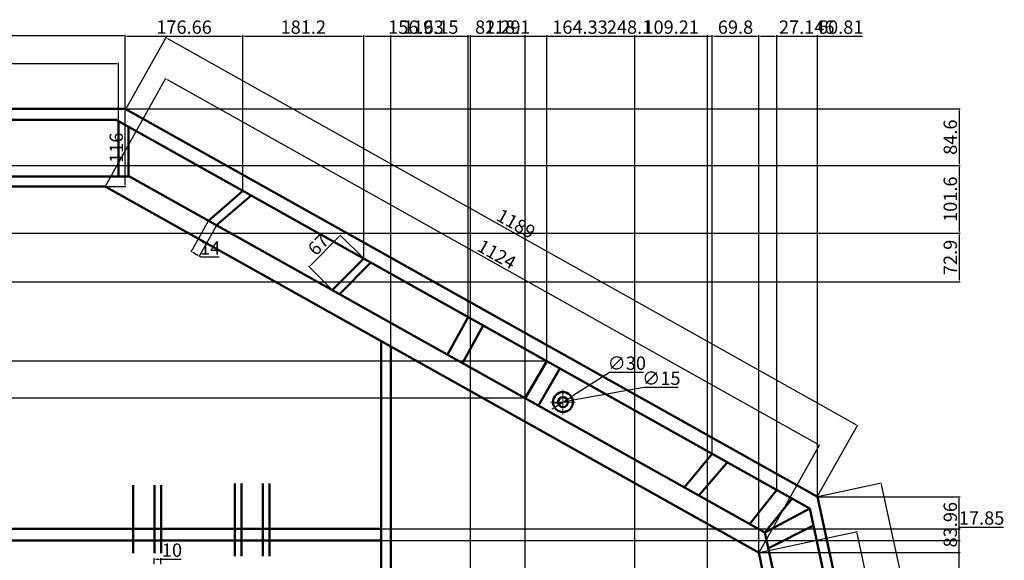
# Model space of a CAD drawing. Units: millimetres. Extents: x 1408 to 3734, y 1022 to 2569.
# Tile 3 of 3: x 2256 to 3734, y 1758 to 2569. Entities that reach past the tile are written whole.
import ezdxf

# ---------------------------------------------------------------- set-up
doc = ezdxf.new("R2010")
doc.units = ezdxf.units.MM
doc.linetypes.add('CENTER2', pattern=[28.575, 19.05, -3.175, 3.175, -3.175])
for name, color, linetype, lineweight in [('M-CNTR', 1, 'CENTER2', 18), ('M-DIMS', 2, 'Continuous', 25), ('M-OUTL', 7, 'Continuous', 50)]:
    doc.layers.add(name, color=color, linetype=linetype, lineweight=lineweight)
doc.styles.get("Standard").update_dxf_attribs({"font": 'arial.ttf'})
doc.dimstyles.new('ISO-25', dxfattribs={"dimtxt": 20, "dimasz": 2.5, "dimexe": 1.25, "dimexo": 0.625, "dimtad": 1, "dimtoh": 1, "dimdec": 0, "dimtxsty": 'Standard', "dimcen": 2.5, "dimadec": 0, "dimazin": 0, "dimtfac": 1, "dimtdec": 0, "dimtmove": 0, "dimatfit": 3, "dimfxl": 1, "dimarcsym": 0})

# ---------------------------------------------------------------- blocks, each defined once
blk = doc.blocks.new('*U1')
at = {"layer": 'M-CNTR', "color": 0, "transparency": 16777216}
for p, q in [((-11, 0), (-1.5, 0)), ((0, 1.5), (0, 11)), ((1.5, 0), (11, 0)), ((0, -11), (0, -1.5))]:
    blk.add_line(p, q, dxfattribs=at)
at = {"layer": 'M-CNTR', "color": 0, "linetype": 'Continuous', "transparency": 16777216}
for p, q in [((-0.7, 0), (0.7, 0)), ((0, -0.7), (0, 0.7))]:
    blk.add_line(p, q, dxfattribs=at)
blk = doc.blocks.new('*U2')
at = {"layer": 'M-CNTR', "color": 0, "transparency": 16777216}
for p, q in [((0, 3), (0, 18.5)), ((-18.5, 0), (-3, 0)), ((3, 0), (18.5, 0)), ((0, -18.5), (0, -3))]:
    blk.add_line(p, q, dxfattribs=at)
at = {"layer": 'M-CNTR', "color": 0, "linetype": 'Continuous', "transparency": 16777216}
for p, q in [((-1.5, 0), (1.5, 0)), ((0, -1.5), (0, 1.5))]:
    blk.add_line(p, q, dxfattribs=at)
blk = doc.blocks.new('*D10')
at = {"layer": 'Defpoints', "color": 0, "transparency": 16777216}
for p in [(2414.7, 2435.4), (2414.7, 2435.4), (2384.8, 2318.9)]:
    blk.add_point(p, dxfattribs=at)
at = {"layer": 'M-DIMS', "color": 0, "lineweight": -2, "transparency": 16777216}
for p, q in [((2414.7, 2321.4), (2414.7, 2432.9)), ((2415.3, 2435.4), (2415.9, 2435.4)), ((2385.4, 2318.9), (2415.9, 2318.9))]:
    blk.add_line(p, q, dxfattribs=at)
at = {"layer": 'M-DIMS', "color": 0, "transparency": 16777216}
for points in [[(2414.3, 2432.9), (2415.1, 2432.9), (2414.7, 2435.4)], [(2414.3, 2321.4), (2415.1, 2321.4), (2414.7, 2318.9)]]:
    blk.add_solid(points, dxfattribs=at)
at = {"layer": 'M-DIMS', "color": 0, "transparency": 16777216, "insert": (2403.9, 2377.2), "char_height": 20, "attachment_point": 5, "rotation": 90}
blk.add_mtext('116', dxfattribs=at)
blk = doc.blocks.new('*D11')
at = {"layer": 'Defpoints', "color": 0, "transparency": 16777216}
for p in [(2415.9, 2435.4), (3513.1, 1960.8), (3453.1, 1853.8)]:
    blk.add_point(p, dxfattribs=at)
at = {"layer": 'M-DIMS', "color": 0, "lineweight": -2, "transparency": 16777216}
for p, q in [((2416.3, 2435.9), (2476.5, 2543.4)), ((2478.1, 2541.1), (3510.9, 1962)), ((3453.4, 1854.4), (3513.7, 1961.8))]:
    blk.add_line(p, q, dxfattribs=at)
at = {"layer": 'M-DIMS', "color": 0, "transparency": 16777216}
for points in [[(2478.3, 2541.4), (2477.9, 2540.7), (2475.9, 2542.3)], [(3511.1, 1962.3), (3510.7, 1961.6), (3513.1, 1960.8)]]:
    blk.add_solid(points, dxfattribs=at)
at = {"layer": 'M-DIMS', "color": 0, "transparency": 16777216, "insert": (2999.8, 2261), "char_height": 20, "attachment_point": 5, "rotation": 330.7202}
blk.add_mtext('1189', dxfattribs=at)
blk = doc.blocks.new('*D12')
at = {"layer": 'Defpoints', "color": 0, "transparency": 16777216}
for p in [(3453.1, 1853.8), (3648.6, 1410), (3553.5, 1389.5)]:
    blk.add_point(p, dxfattribs=at)
at = {"layer": 'M-DIMS', "color": 0, "lineweight": -2, "transparency": 16777216}
for p, q in [((3453.7, 1854), (3549.5, 1874.7)), ((3548.8, 1871.9), (3648.1, 1412.5)), ((3554.1, 1389.6), (3649.8, 1410.3))]:
    blk.add_line(p, q, dxfattribs=at)
at = {"layer": 'M-DIMS', "color": 0, "transparency": 16777216}
for points in [[(3549.2, 1872), (3548.4, 1871.9), (3548.3, 1874.4)], [(3648.5, 1412.6), (3647.7, 1412.4), (3648.6, 1410)]]:
    blk.add_solid(points, dxfattribs=at)
at = {"layer": 'M-DIMS', "color": 0, "transparency": 16777216, "insert": (3609, 1644.5), "char_height": 20, "attachment_point": 5, "rotation": 282.1929}
blk.add_mtext('475', dxfattribs=at)
blk = doc.blocks.new('*D13')
at = {"layer": 'Defpoints', "color": 0, "transparency": 16777216}
for p in [(1964.7, 2545.3), (1964.7, 2435.4), (2414.7, 2435.4)]:
    blk.add_point(p, dxfattribs=at)
at = {"layer": 'M-DIMS', "color": 0, "lineweight": -2, "transparency": 16777216}
for p, q in [((1964.7, 2436), (1964.7, 2546.6)), ((2412.2, 2545.3), (1967.2, 2545.3)), ((2414.7, 2436), (2414.7, 2546.6))]:
    blk.add_line(p, q, dxfattribs=at)
at = {"layer": 'M-DIMS', "color": 0, "transparency": 16777216}
for points in [[(1967.2, 2545.7), (1967.2, 2544.9), (1964.7, 2545.3)], [(2412.2, 2545.7), (2412.2, 2544.9), (2414.7, 2545.3)]]:
    blk.add_solid(points, dxfattribs=at)
at = {"layer": 'M-DIMS', "color": 0, "transparency": 16777216, "insert": (2189.7, 2556.1), "char_height": 20, "attachment_point": 5}
blk.add_mtext('450', dxfattribs=at)
blk = doc.blocks.new('*D15')
at = {"layer": 'Defpoints', "color": 0, "transparency": 16777216}
for p in [(2468.4, 1760.2), (2458.4, 1752.1), (2468.4, 1752.1)]:
    blk.add_point(p, dxfattribs=at)
at = {"layer": 'M-DIMS', "color": 0, "lineweight": -2, "transparency": 16777216}
for p, q in [((2458.4, 1752.7), (2458.4, 1761.5)), ((2460.9, 1760.2), (2465.9, 1760.2)), ((2468.4, 1752.7), (2468.4, 1761.5)), ((2468.4, 1760.2), (2498.9, 1760.2))]:
    blk.add_line(p, q, dxfattribs=at)
at = {"layer": 'M-DIMS', "color": 0, "transparency": 16777216}
for points in [[(2460.9, 1760.6), (2460.9, 1759.8), (2458.4, 1760.2)], [(2465.9, 1760.6), (2465.9, 1759.8), (2468.4, 1760.2)]]:
    blk.add_solid(points, dxfattribs=at)
at = {"layer": 'M-DIMS', "color": 0, "transparency": 16777216, "insert": (2484.9, 1771), "char_height": 20, "attachment_point": 5}
blk.add_mtext('10', dxfattribs=at)
blk = doc.blocks.new('*D18')
at = {"layer": 'Defpoints', "color": 0, "transparency": 16777216}
for p in [(3084.1, 2003.7), (3058.8, 1987.7)]:
    blk.add_point(p, dxfattribs=at)
at = {"layer": 'M-DIMS', "color": 0, "lineweight": -2, "transparency": 16777216}
for p, q in [((3141.4, 2040.1), (3086.2, 2005.1)), ((3192.3, 2040.1), (3141.4, 2040.1)), ((3058.8, 1987.7), (3084.1, 2003.7)), ((3056.7, 1986.3), (3054.6, 1985))]:
    blk.add_line(p, q, dxfattribs=at)
at = {"layer": 'M-DIMS', "color": 0, "transparency": 16777216}
for points in [[(3086, 2005.4), (3086.4, 2004.7), (3084.1, 2003.7)], [(3056.5, 1986.7), (3056.9, 1986), (3058.8, 1987.7)]]:
    blk.add_solid(points, dxfattribs=at)
at = {"layer": 'M-DIMS', "color": 0, "transparency": 16777216, "insert": (3167.2, 2051.5), "char_height": 20, "attachment_point": 5}
blk.add_mtext('∅30', dxfattribs=at)
blk = doc.blocks.new('*D19')
at = {"layer": 'Defpoints', "color": 0, "transparency": 16777216}
for p in [(3064.1, 1994.4), (3078.8, 1997)]:
    blk.add_point(p, dxfattribs=at)
at = {"layer": 'M-DIMS', "color": 0, "lineweight": -2, "transparency": 16777216}
for p, q in [((3193, 2017.5), (3081.3, 1997.5)), ((3244.2, 2017.5), (3193, 2017.5)), ((3064.1, 1994.4), (3078.8, 1997)), ((3061.6, 1993.9), (3059.1, 1993.5))]:
    blk.add_line(p, q, dxfattribs=at)
at = {"layer": 'M-DIMS', "color": 0, "transparency": 16777216}
for points in [[(3061.5, 1994.3), (3061.7, 1993.5), (3064.1, 1994.4)], [(3081.2, 1997.9), (3081.4, 1997.1), (3078.8, 1997)]]:
    blk.add_solid(points, dxfattribs=at)
at = {"layer": 'M-DIMS', "color": 0, "transparency": 16777216, "insert": (3219, 2028.9), "char_height": 20, "attachment_point": 5}
blk.add_mtext('∅15', dxfattribs=at)
blk = doc.blocks.new('*D25')
at = {"layer": 'Defpoints', "color": 0, "transparency": 16777216}
for p in [(2539.7, 2267.8), (2551.9, 2260.9), (2526.1, 2214.8)]:
    blk.add_point(p, dxfattribs=at)
at = {"layer": 'M-DIMS', "color": 0, "lineweight": -2, "transparency": 16777216}
for p, q in [((2539.4, 2267.2), (2513.2, 2220.6)), ((2551.6, 2260.4), (2525.4, 2213.7)), ((2516, 2220.4), (2523.9, 2216)), ((2526.1, 2214.8), (2528.2, 2213.6)), ((2528.2, 2213.6), (2555.5, 2213.6))]:
    blk.add_line(p, q, dxfattribs=at)
at = {"layer": 'M-DIMS', "color": 0, "transparency": 16777216}
for points in [[(2516.2, 2220.8), (2515.8, 2220.1), (2513.8, 2221.6)], [(2524.1, 2216.4), (2523.7, 2215.7), (2526.1, 2214.8)]]:
    blk.add_solid(points, dxfattribs=at)
at = {"layer": 'M-DIMS', "color": 0, "transparency": 16777216, "insert": (2542.2, 2224.3), "char_height": 20, "attachment_point": 5}
blk.add_mtext('14', dxfattribs=at)
blk = doc.blocks.new('*D27')
at = {"layer": 'Defpoints', "color": 0, "transparency": 16777216}
for p in [(2384.8, 2318.9), (3456.2, 1931.2), (3365.6, 1769.6)]:
    blk.add_point(p, dxfattribs=at)
at = {"layer": 'M-DIMS', "color": 0, "lineweight": -2, "transparency": 16777216}
for p, q in [((2385.1, 2319.5), (2475.9, 2481.7)), ((2477.5, 2479.4), (3454, 1932.5)), ((3365.9, 1770.1), (3456.8, 1932.3))]:
    blk.add_line(p, q, dxfattribs=at)
at = {"layer": 'M-DIMS', "color": 0, "transparency": 16777216}
for points in [[(2477.7, 2479.7), (2477.3, 2479), (2475.3, 2480.6)], [(3454.2, 1932.8), (3453.8, 1932.1), (3456.2, 1931.2)]]:
    blk.add_solid(points, dxfattribs=at)
at = {"layer": 'M-DIMS', "color": 0, "transparency": 16777216, "insert": (2970.9, 2215.2), "char_height": 20, "attachment_point": 5, "rotation": 330.7496}
blk.add_mtext('1124', dxfattribs=at)
blk = doc.blocks.new('*D28')
at = {"layer": 'Defpoints', "color": 0, "transparency": 16777216}
for p in [(3365.2, 1769.9), (3598.5, 1400), (3451.8, 1368.3)]:
    blk.add_point(p, dxfattribs=at)
at = {"layer": 'M-DIMS', "color": 0, "lineweight": -2, "transparency": 16777216}
for p, q in [((3365.8, 1770), (3513.1, 1801.8)), ((3512.4, 1799.1), (3598, 1402.4)), ((3452.4, 1368.4), (3599.8, 1400.2))]:
    blk.add_line(p, q, dxfattribs=at)
at = {"layer": 'M-DIMS', "color": 0, "transparency": 16777216}
for points in [[(3512.8, 1799.2), (3512, 1799), (3511.9, 1801.5)], [(3598.4, 1402.5), (3597.6, 1402.3), (3598.5, 1400)]]:
    blk.add_solid(points, dxfattribs=at)
at = {"layer": 'M-DIMS', "color": 0, "transparency": 16777216, "insert": (3565.6, 1603), "char_height": 20, "attachment_point": 5, "rotation": 282.179}
blk.add_mtext('411', dxfattribs=at)
blk = doc.blocks.new('*D34')
at = {"layer": 'Defpoints', "color": 0, "transparency": 16777216}
for p in [(1980.7, 2503.2), (1980.7, 2418.9), (2404.5, 2417.1)]:
    blk.add_point(p, dxfattribs=at)
at = {"layer": 'M-DIMS', "color": 0, "lineweight": -2, "transparency": 16777216}
for p, q in [((1980.7, 2419.6), (1980.7, 2504.4)), ((2402, 2503.2), (1983.2, 2503.2)), ((2404.5, 2417.7), (2404.5, 2504.4))]:
    blk.add_line(p, q, dxfattribs=at)
at = {"layer": 'M-DIMS', "color": 0, "transparency": 16777216}
for points in [[(1983.2, 2503.6), (1983.2, 2502.8), (1980.7, 2503.2)], [(2402, 2503.6), (2402, 2502.8), (2404.5, 2503.2)]]:
    blk.add_solid(points, dxfattribs=at)
at = {"layer": 'M-DIMS', "color": 0, "transparency": 16777216, "insert": (2192.6, 2513.8), "char_height": 20, "attachment_point": 5}
blk.add_mtext('424', dxfattribs=at)
blk = doc.blocks.new('*D37')
at = {"layer": 'Defpoints', "color": 0, "transparency": 16777216}
for p in [(2737.4, 2245.8), (2772.5, 2210.9), (2725.6, 2163.6)]:
    blk.add_point(p, dxfattribs=at)
at = {"layer": 'M-DIMS', "color": 0, "lineweight": -2, "transparency": 16777216}
for p, q in [((2772.1, 2211.4), (2736.5, 2246.7)), ((2692.2, 2200.3), (2735.6, 2244)), ((2725.2, 2164.1), (2689.6, 2199.4))]:
    blk.add_line(p, q, dxfattribs=at)
at = {"layer": 'M-DIMS', "color": 0, "transparency": 16777216}
for points in [[(2735.3, 2244.3), (2735.9, 2243.7), (2737.4, 2245.8)], [(2691.9, 2200.5), (2692.5, 2200), (2690.5, 2198.5)]]:
    blk.add_solid(points, dxfattribs=at)
at = {"layer": 'M-DIMS', "color": 0, "transparency": 16777216, "insert": (2706.2, 2229.8), "char_height": 20, "attachment_point": 5, "rotation": 45.239}
blk.add_mtext('67', dxfattribs=at)
blk = doc.blocks.new('*D42')
at = {"layer": 'Defpoints', "color": 0, "transparency": 16777216}
for p in [(1677, 2435.4), (1671.8, 2350.8), (3665.9, 2350.8)]:
    blk.add_point(p, dxfattribs=at)
at = {"layer": 'M-DIMS', "color": 0, "lineweight": -2, "transparency": 16777216}
for p, q in [((1677.6, 2435.4), (3667.2, 2435.4)), ((3665.9, 2432.9), (3665.9, 2353.3)), ((1672.5, 2350.8), (3667.2, 2350.8))]:
    blk.add_line(p, q, dxfattribs=at)
at = {"layer": 'M-DIMS', "color": 0, "transparency": 16777216}
for points in [[(3665.5, 2432.9), (3666.4, 2432.9), (3665.9, 2435.4)], [(3665.5, 2353.3), (3666.4, 2353.3), (3665.9, 2350.8)]]:
    blk.add_solid(points, dxfattribs=at)
at = {"layer": 'M-DIMS', "color": 0, "transparency": 16777216, "insert": (3655.1, 2393.1), "char_height": 20, "attachment_point": 5, "rotation": 90}
blk.add_mtext('84.6', dxfattribs=at)
blk = doc.blocks.new('*D43')
at = {"layer": 'Defpoints', "color": 0, "transparency": 16777216}
for p in [(1671.8, 2350.8), (1671.8, 2249.2), (3665.9, 2249.2)]:
    blk.add_point(p, dxfattribs=at)
at = {"layer": 'M-DIMS', "color": 0, "lineweight": -2, "transparency": 16777216}
for p, q in [((1672.5, 2350.8), (3667.2, 2350.8)), ((3665.9, 2348.3), (3665.9, 2251.7)), ((1672.5, 2249.2), (3667.2, 2249.2))]:
    blk.add_line(p, q, dxfattribs=at)
at = {"layer": 'M-DIMS', "color": 0, "transparency": 16777216}
for points in [[(3665.5, 2348.3), (3666.4, 2348.3), (3665.9, 2350.8)], [(3665.5, 2251.7), (3666.4, 2251.7), (3665.9, 2249.2)]]:
    blk.add_solid(points, dxfattribs=at)
at = {"layer": 'M-DIMS', "color": 0, "transparency": 16777216, "insert": (3655.1, 2300), "char_height": 20, "attachment_point": 5, "rotation": 90}
blk.add_mtext('101.6', dxfattribs=at)
blk = doc.blocks.new('*D44')
at = {"layer": 'Defpoints', "color": 0, "transparency": 16777216}
for p in [(1671.8, 2249.2), (1671.8, 2176.3), (3665.9, 2176.3)]:
    blk.add_point(p, dxfattribs=at)
at = {"layer": 'M-DIMS', "color": 0, "lineweight": -2, "transparency": 16777216}
for p, q in [((1672.5, 2249.2), (3667.2, 2249.2)), ((3665.9, 2246.7), (3665.9, 2178.8)), ((1672.5, 2176.3), (3667.2, 2176.3))]:
    blk.add_line(p, q, dxfattribs=at)
at = {"layer": 'M-DIMS', "color": 0, "transparency": 16777216}
for points in [[(3665.5, 2246.7), (3666.4, 2246.7), (3665.9, 2249.2)], [(3665.5, 2178.8), (3666.4, 2178.8), (3665.9, 2176.3)]]:
    blk.add_solid(points, dxfattribs=at)
at = {"layer": 'M-DIMS', "color": 0, "transparency": 16777216, "insert": (3655.1, 2212.7), "char_height": 20, "attachment_point": 5, "rotation": 90}
blk.add_mtext('72.9', dxfattribs=at)
blk = doc.blocks.new('*D50')
at = {"layer": 'Defpoints', "color": 0, "transparency": 16777216}
for p in [(1475.7, 2057.1), (3047.3, 2057.1), (3014.5, 2001.8)]:
    blk.add_point(p, dxfattribs=at)
at = {"layer": 'M-DIMS', "color": 0, "lineweight": -2, "transparency": 16777216}
for p, q in [((3046.6, 2057.1), (1474.5, 2057.1)), ((1475.7, 2057.1), (1475.7, 2059.6)), ((1475.7, 2059.6), (1543.8, 2059.6)), ((1475.7, 2004.3), (1475.7, 2054.6)), ((3013.9, 2001.8), (1474.5, 2001.8))]:
    blk.add_line(p, q, dxfattribs=at)
at = {"layer": 'M-DIMS', "color": 0, "transparency": 16777216}
for points in [[(1475.3, 2054.6), (1476.1, 2054.6), (1475.7, 2057.1)], [(1475.3, 2004.3), (1476.1, 2004.3), (1475.7, 2001.8)]]:
    blk.add_solid(points, dxfattribs=at)
at = {"layer": 'M-DIMS', "color": 0, "transparency": 16777216, "insert": (1510.1, 2070.4), "char_height": 20, "attachment_point": 5}
blk.add_mtext('55.27', dxfattribs=at)
blk = doc.blocks.new('*D51')
at = {"layer": 'Defpoints', "color": 0, "transparency": 16777216}
for p in [(3365.2, 1769.9), (3665.9, 1769.9), (3556.7, 1373.9)]:
    blk.add_point(p, dxfattribs=at)
at = {"layer": 'M-DIMS', "color": 0, "lineweight": -2, "transparency": 16777216}
for p, q in [((3365.8, 1769.9), (3667.2, 1769.9)), ((3665.9, 1376.4), (3665.9, 1767.4)), ((3557.3, 1373.9), (3667.2, 1373.9))]:
    blk.add_line(p, q, dxfattribs=at)
at = {"layer": 'M-DIMS', "color": 0, "transparency": 16777216}
for points in [[(3665.5, 1767.4), (3666.4, 1767.4), (3665.9, 1769.9)], [(3665.5, 1376.4), (3666.4, 1376.4), (3665.9, 1373.9)]]:
    blk.add_solid(points, dxfattribs=at)
at = {"layer": 'M-DIMS', "color": 0, "transparency": 16777216, "insert": (3655.1, 1571.9), "char_height": 20, "attachment_point": 5, "rotation": 90}
blk.add_mtext('396', dxfattribs=at)
blk = doc.blocks.new('*D52')
at = {"layer": 'Defpoints', "color": 0, "transparency": 16777216}
for p in [(3453.1, 1853.8), (3665.9, 1853.8), (3365.2, 1769.9)]:
    blk.add_point(p, dxfattribs=at)
at = {"layer": 'M-DIMS', "color": 0, "lineweight": -2, "transparency": 16777216}
for p, q in [((3453.7, 1853.8), (3667.2, 1853.8)), ((3665.9, 1772.4), (3665.9, 1851.3)), ((3365.8, 1769.9), (3667.2, 1769.9))]:
    blk.add_line(p, q, dxfattribs=at)
at = {"layer": 'M-DIMS', "color": 0, "transparency": 16777216}
for points in [[(3665.5, 1851.3), (3666.4, 1851.3), (3665.9, 1853.8)], [(3665.5, 1772.4), (3666.4, 1772.4), (3665.9, 1769.9)]]:
    blk.add_solid(points, dxfattribs=at)
at = {"layer": 'M-DIMS', "color": 0, "transparency": 16777216, "insert": (3655.1, 1811.8), "char_height": 20, "attachment_point": 5, "rotation": 90}
blk.add_mtext('83.96', dxfattribs=at)
blk = doc.blocks.new('*D56')
at = {"layer": 'Defpoints', "color": 0, "transparency": 16777216}
for p in [(2798.6, 1805.8), (3665.9, 1805.8), (2813.4, 1235.4)]:
    blk.add_point(p, dxfattribs=at)
at = {"layer": 'M-DIMS', "color": 0, "lineweight": -2, "transparency": 16777216}
for p, q in [((2799.2, 1805.8), (3667.2, 1805.8)), ((3665.9, 1237.9), (3665.9, 1803.3)), ((2814.1, 1235.4), (3667.2, 1235.4))]:
    blk.add_line(p, q, dxfattribs=at)
at = {"layer": 'M-DIMS', "color": 0, "transparency": 16777216}
for points in [[(3665.5, 1803.3), (3666.4, 1803.3), (3665.9, 1805.8)], [(3665.5, 1237.9), (3666.4, 1237.9), (3665.9, 1235.4)]]:
    blk.add_solid(points, dxfattribs=at)
at = {"layer": 'M-DIMS', "color": 0, "transparency": 16777216, "insert": (3655.1, 1520.6), "char_height": 20, "attachment_point": 5, "rotation": 90}
blk.add_mtext('570.4', dxfattribs=at)
blk = doc.blocks.new('*D57')
at = {"layer": 'Defpoints', "color": 0, "transparency": 16777216}
for p in [(2798.6, 1805.8), (3665.9, 1805.8), (2798.6, 1788)]:
    blk.add_point(p, dxfattribs=at)
at = {"layer": 'M-DIMS', "color": 0, "lineweight": -2, "transparency": 16777216}
for p, q in [((2799.2, 1805.8), (3667.2, 1805.8)), ((3665.9, 1805.8), (3665.9, 1808.3)), ((3665.9, 1808.3), (3732.3, 1808.3)), ((3665.9, 1790.5), (3665.9, 1803.3)), ((2799.2, 1788), (3667.2, 1788))]:
    blk.add_line(p, q, dxfattribs=at)
at = {"layer": 'M-DIMS', "color": 0, "transparency": 16777216}
for points in [[(3665.5, 1803.3), (3666.4, 1803.3), (3665.9, 1805.8)], [(3665.5, 1790.5), (3666.4, 1790.5), (3665.9, 1788)]]:
    blk.add_solid(points, dxfattribs=at)
at = {"layer": 'M-DIMS', "color": 0, "transparency": 16777216, "insert": (3699.5, 1819.2), "char_height": 20, "attachment_point": 5}
blk.add_mtext('17.85', dxfattribs=at)
blk = doc.blocks.new('*D67')
at = {"layer": 'Defpoints', "color": 0, "transparency": 16777216}
for p in [(2591.4, 2544.6), (2414.7, 2435.4), (2591.4, 2312.4)]:
    blk.add_point(p, dxfattribs=at)
at = {"layer": 'M-DIMS', "color": 0, "lineweight": -2, "transparency": 16777216}
for p, q in [((2414.7, 2436), (2414.7, 2545.9)), ((2417.2, 2544.6), (2588.9, 2544.6)), ((2591.4, 2313), (2591.4, 2545.9))]:
    blk.add_line(p, q, dxfattribs=at)
at = {"layer": 'M-DIMS', "color": 0, "transparency": 16777216}
for points in [[(2417.2, 2545), (2417.2, 2544.2), (2414.7, 2544.6)], [(2588.9, 2545), (2588.9, 2544.2), (2591.4, 2544.6)]]:
    blk.add_solid(points, dxfattribs=at)
at = {"layer": 'M-DIMS', "color": 0, "transparency": 16777216, "insert": (2503, 2555.5), "char_height": 20, "attachment_point": 5}
blk.add_mtext('176.66', dxfattribs=at)
blk = doc.blocks.new('*D68')
at = {"layer": 'Defpoints', "color": 0, "transparency": 16777216}
for p in [(2772.5, 2544.6), (2591.4, 2312.4), (2772.5, 2210.9)]:
    blk.add_point(p, dxfattribs=at)
at = {"layer": 'M-DIMS', "color": 0, "lineweight": -2, "transparency": 16777216}
for p, q in [((2591.4, 2313), (2591.4, 2545.9)), ((2593.9, 2544.6), (2770, 2544.6)), ((2772.5, 2211.6), (2772.5, 2545.9))]:
    blk.add_line(p, q, dxfattribs=at)
at = {"layer": 'M-DIMS', "color": 0, "transparency": 16777216}
for points in [[(2593.9, 2545), (2593.9, 2544.2), (2591.4, 2544.6)], [(2770, 2545), (2770, 2544.2), (2772.5, 2544.6)]]:
    blk.add_solid(points, dxfattribs=at)
at = {"layer": 'M-DIMS', "color": 0, "transparency": 16777216, "insert": (2681.9, 2555.5), "char_height": 20, "attachment_point": 5}
blk.add_mtext('181.2', dxfattribs=at)
blk = doc.blocks.new('*D69')
at = {"layer": 'Defpoints', "color": 0, "transparency": 16777216}
for p in [(2929.2, 2544.6), (2772.5, 2210.9), (2929.2, 2123.2)]:
    blk.add_point(p, dxfattribs=at)
at = {"layer": 'M-DIMS', "color": 0, "lineweight": -2, "transparency": 16777216}
for p, q in [((2772.5, 2211.6), (2772.5, 2545.9)), ((2775, 2544.6), (2926.7, 2544.6)), ((2929.2, 2123.9), (2929.2, 2545.9))]:
    blk.add_line(p, q, dxfattribs=at)
at = {"layer": 'M-DIMS', "color": 0, "transparency": 16777216}
for points in [[(2775, 2545), (2775, 2544.2), (2772.5, 2544.6)], [(2926.7, 2545), (2926.7, 2544.2), (2929.2, 2544.6)]]:
    blk.add_solid(points, dxfattribs=at)
at = {"layer": 'M-DIMS', "color": 0, "transparency": 16777216, "insert": (2850.9, 2555.5), "char_height": 20, "attachment_point": 5}
blk.add_mtext('156.63', dxfattribs=at)
blk = doc.blocks.new('*D70')
at = {"layer": 'Defpoints', "color": 0, "transparency": 16777216}
for p in [(3047.3, 2544.6), (2929.2, 2123.2), (3047.3, 2057.1)]:
    blk.add_point(p, dxfattribs=at)
at = {"layer": 'M-DIMS', "color": 0, "lineweight": -2, "transparency": 16777216}
for p, q in [((2929.2, 2123.9), (2929.2, 2545.9)), ((2931.7, 2544.6), (3044.8, 2544.6)), ((3047.3, 2057.7), (3047.3, 2545.9))]:
    blk.add_line(p, q, dxfattribs=at)
at = {"layer": 'M-DIMS', "color": 0, "transparency": 16777216}
for points in [[(2931.7, 2545), (2931.7, 2544.2), (2929.2, 2544.6)], [(3044.8, 2545), (3044.8, 2544.2), (3047.3, 2544.6)]]:
    blk.add_solid(points, dxfattribs=at)
at = {"layer": 'M-DIMS', "color": 0, "transparency": 16777216, "insert": (2988.2, 2555.5), "char_height": 20, "attachment_point": 5}
blk.add_mtext('118.1', dxfattribs=at)
blk = doc.blocks.new('*D71')
at = {"layer": 'Defpoints', "color": 0, "transparency": 16777216}
for p in [(3295.4, 2544.6), (3047.3, 2057.1), (3295.4, 1918.2)]:
    blk.add_point(p, dxfattribs=at)
at = {"layer": 'M-DIMS', "color": 0, "lineweight": -2, "transparency": 16777216}
for p, q in [((3047.3, 2057.7), (3047.3, 2545.9)), ((3049.8, 2544.6), (3292.9, 2544.6)), ((3295.4, 1918.8), (3295.4, 2545.9))]:
    blk.add_line(p, q, dxfattribs=at)
at = {"layer": 'M-DIMS', "color": 0, "transparency": 16777216}
for points in [[(3049.8, 2545), (3049.8, 2544.2), (3047.3, 2544.6)], [(3292.9, 2545), (3292.9, 2544.2), (3295.4, 2544.6)]]:
    blk.add_solid(points, dxfattribs=at)
at = {"layer": 'M-DIMS', "color": 0, "transparency": 16777216, "insert": (3171.3, 2555.5), "char_height": 20, "attachment_point": 5}
blk.add_mtext('248.1', dxfattribs=at)
blk = doc.blocks.new('*D72')
at = {"layer": 'Defpoints', "color": 0, "transparency": 16777216}
for p in [(3365.2, 2544.6), (3295.4, 1918.2), (3365.2, 1769.9)]:
    blk.add_point(p, dxfattribs=at)
at = {"layer": 'M-DIMS', "color": 0, "lineweight": -2, "transparency": 16777216}
for p, q in [((3295.4, 1918.8), (3295.4, 2545.9)), ((3297.9, 2544.6), (3362.7, 2544.6)), ((3365.2, 1770.5), (3365.2, 2545.9))]:
    blk.add_line(p, q, dxfattribs=at)
at = {"layer": 'M-DIMS', "color": 0, "transparency": 16777216}
for points in [[(3297.9, 2545), (3297.9, 2544.2), (3295.4, 2544.6)], [(3362.7, 2545), (3362.7, 2544.2), (3365.2, 2544.6)]]:
    blk.add_solid(points, dxfattribs=at)
at = {"layer": 'M-DIMS', "color": 0, "transparency": 16777216, "insert": (3330.3, 2555.5), "char_height": 20, "attachment_point": 5}
blk.add_mtext('69.8', dxfattribs=at)
blk = doc.blocks.new('*D73')
at = {"layer": 'Defpoints', "color": 0, "transparency": 16777216}
for p in [(3392.3, 2544.6), (3392.3, 1863.9), (3365.2, 1769.9)]:
    blk.add_point(p, dxfattribs=at)
at = {"layer": 'M-DIMS', "color": 0, "lineweight": -2, "transparency": 16777216}
for p, q in [((3365.2, 1770.5), (3365.2, 2545.9)), ((3367.7, 2544.6), (3389.8, 2544.6)), ((3392.3, 1864.5), (3392.3, 2545.9)), ((3392.3, 2544.6), (3479.4, 2544.6))]:
    blk.add_line(p, q, dxfattribs=at)
at = {"layer": 'M-DIMS', "color": 0, "transparency": 16777216}
for points in [[(3367.7, 2545), (3367.7, 2544.2), (3365.2, 2544.6)], [(3389.8, 2545), (3389.8, 2544.2), (3392.3, 2544.6)]]:
    blk.add_solid(points, dxfattribs=at)
at = {"layer": 'M-DIMS', "color": 0, "transparency": 16777216, "insert": (3437.1, 2555.5), "char_height": 20, "attachment_point": 5}
blk.add_mtext('27.146', dxfattribs=at)
blk = doc.blocks.new('*D74')
at = {"layer": 'Defpoints', "color": 0, "transparency": 16777216}
for p in [(3453.1, 2544.6), (3392.3, 1863.9), (3453.1, 1853.8)]:
    blk.add_point(p, dxfattribs=at)
at = {"layer": 'M-DIMS', "color": 0, "lineweight": -2, "transparency": 16777216}
for p, q in [((3392.3, 1864.5), (3392.3, 2545.9)), ((3394.8, 2544.6), (3450.6, 2544.6)), ((3453.1, 1854.5), (3453.1, 2545.9)), ((3453.1, 2544.6), (3520.6, 2544.6))]:
    blk.add_line(p, q, dxfattribs=at)
at = {"layer": 'M-DIMS', "color": 0, "transparency": 16777216}
for points in [[(3394.8, 2545), (3394.8, 2544.2), (3392.3, 2544.6)], [(3450.6, 2545), (3450.6, 2544.2), (3453.1, 2544.6)]]:
    blk.add_solid(points, dxfattribs=at)
at = {"layer": 'M-DIMS', "color": 0, "transparency": 16777216, "insert": (3488.1, 2555.5), "char_height": 20, "attachment_point": 5}
blk.add_mtext('60.81', dxfattribs=at)
blk = doc.blocks.new('*D77')
at = {"layer": 'Defpoints', "color": 0, "transparency": 16777216}
for p in [(2932.6, 2544.6), (2932.6, 1367.8), (2813.4, 1235.4)]:
    blk.add_point(p, dxfattribs=at)
at = {"layer": 'M-DIMS', "color": 0, "lineweight": -2, "transparency": 16777216}
for p, q in [((2813.4, 1236), (2813.4, 2545.9)), ((2815.9, 2544.6), (2930.1, 2544.6)), ((2932.6, 1368.4), (2932.6, 2545.9))]:
    blk.add_line(p, q, dxfattribs=at)
at = {"layer": 'M-DIMS', "color": 0, "transparency": 16777216}
for points in [[(2815.9, 2545), (2815.9, 2544.2), (2813.4, 2544.6)], [(2930.1, 2545), (2930.1, 2544.2), (2932.6, 2544.6)]]:
    blk.add_solid(points, dxfattribs=at)
at = {"layer": 'M-DIMS', "color": 0, "transparency": 16777216, "insert": (2873, 2555.5), "char_height": 20, "attachment_point": 5}
blk.add_mtext('119.15', dxfattribs=at)
blk = doc.blocks.new('*D78')
at = {"layer": 'Defpoints', "color": 0, "transparency": 16777216}
for p in [(3014.9, 2544.6), (3014.9, 1392.8), (2932.6, 1367.8)]:
    blk.add_point(p, dxfattribs=at)
at = {"layer": 'M-DIMS', "color": 0, "lineweight": -2, "transparency": 16777216}
for p, q in [((2932.6, 1368.4), (2932.6, 2545.9)), ((2935.1, 2544.6), (3012.4, 2544.6)), ((3014.9, 1393.4), (3014.9, 2545.9))]:
    blk.add_line(p, q, dxfattribs=at)
at = {"layer": 'M-DIMS', "color": 0, "transparency": 16777216}
for points in [[(2935.1, 2545), (2935.1, 2544.2), (2932.6, 2544.6)], [(3012.4, 2545), (3012.4, 2544.2), (3014.9, 2544.6)]]:
    blk.add_solid(points, dxfattribs=at)
at = {"layer": 'M-DIMS', "color": 0, "transparency": 16777216, "insert": (2973.7, 2555.5), "char_height": 20, "attachment_point": 5}
blk.add_mtext('82.29', dxfattribs=at)
blk = doc.blocks.new('*D79')
at = {"layer": 'Defpoints', "color": 0, "transparency": 16777216}
for p in [(3179.2, 2544.6), (3179.2, 1443.7), (3014.9, 1392.8)]:
    blk.add_point(p, dxfattribs=at)
at = {"layer": 'M-DIMS', "color": 0, "lineweight": -2, "transparency": 16777216}
for p, q in [((3014.9, 1393.4), (3014.9, 2545.9)), ((3017.4, 2544.6), (3176.7, 2544.6)), ((3179.2, 1444.3), (3179.2, 2545.9))]:
    blk.add_line(p, q, dxfattribs=at)
at = {"layer": 'M-DIMS', "color": 0, "transparency": 16777216}
for points in [[(3017.4, 2545), (3017.4, 2544.2), (3014.9, 2544.6)], [(3176.7, 2545), (3176.7, 2544.2), (3179.2, 2544.6)]]:
    blk.add_solid(points, dxfattribs=at)
at = {"layer": 'M-DIMS', "color": 0, "transparency": 16777216, "insert": (3097, 2555.5), "char_height": 20, "attachment_point": 5}
blk.add_mtext('164.33', dxfattribs=at)
blk = doc.blocks.new('*D80')
at = {"layer": 'Defpoints', "color": 0, "transparency": 16777216}
for p in [(3288.4, 2544.6), (3288.4, 1477.1), (3179.2, 1443.7)]:
    blk.add_point(p, dxfattribs=at)
at = {"layer": 'M-DIMS', "color": 0, "lineweight": -2, "transparency": 16777216}
for p, q in [((3179.2, 1444.3), (3179.2, 2545.9)), ((3181.7, 2544.6), (3285.9, 2544.6)), ((3288.4, 1477.7), (3288.4, 2545.9))]:
    blk.add_line(p, q, dxfattribs=at)
at = {"layer": 'M-DIMS', "color": 0, "transparency": 16777216}
for points in [[(3181.7, 2545), (3181.7, 2544.2), (3179.2, 2544.6)], [(3285.9, 2545), (3285.9, 2544.2), (3288.4, 2544.6)]]:
    blk.add_solid(points, dxfattribs=at)
at = {"layer": 'M-DIMS', "color": 0, "transparency": 16777216, "insert": (3233.8, 2555.5), "char_height": 20, "attachment_point": 5}
blk.add_mtext('109.21', dxfattribs=at)

msp = doc.modelspace()

# ---------------------------------------------------------------- linework, layer by layer
at = {"layer": 'M-OUTL'}
for p, q in [((1964.6991, 2435.3757), (2414.6991, 2435.3757)), ((2414.6991, 2435.3757), (3422.4282, 1871.0114)), ((1980.6517, 2418.9311), (2401.1247, 2418.9311)), ((2404.4571, 2417.0877), (2401.1247, 2418.9311)), ((2404.4571, 2417.0877), (3412.1862, 1852.7234)), ((2404.4571, 2417.0877), (2404.4571, 2334.2032)), ((2419.6288, 2408.591), (2419.6288, 2334.0442)), ((2092.8085, 2334.2032), (2411.4791, 2334.2032)), ((2411.4791, 2334.2032), (2421.3636, 2334.0104)), ((2421.3636, 2334.0104), (3374.4518, 1800.247)), ((2077.4791, 2318.9311), (2384.7504, 2318.9311)), ((2384.7504, 2318.9311), (3365.6347, 1769.6009)), ((2384.7504, 2318.9311), (3365.6347, 1769.6009)), ((2591.3565, 2312.4174), (2539.6699, 2267.7546)), ((2599.9562, 2302.4652), (2603.4077, 2305.6682)), ((2599.9562, 2302.4652), (2551.876, 2260.9187)), ((2727.9376, 2165.9433), (2772.5401, 2210.9481)), ((2736.3485, 2157.6076), (2783.2616, 2204.9437)), ((2727.9376, 2165.9433), (2725.6079, 2163.6227)), ((2929.1658, 2123.2321), (2898.0885, 2067.0274)), ((2920.8068, 2054.3043), (2951.8378, 2110.5349)), ((2798.6154, 1235.3757), (2798.6154, 2087.152)), ((2813.4357, 1235.3757), (2813.4357, 2078.8521)), ((3047.2723, 2057.0882), (3014.522, 2001.8205)), ((3034.7027, 1990.5186), (3066.9619, 2046.0613)), ((3295.357, 1918.1519), (3253.5096, 1867.9789)), ((3275.3081, 1855.771), (3318.2275, 1905.3436)), ((2426.4129, 1768.9067), (2426.4129, 1870.9323)), ((2458.4129, 1870.9323), (2458.4129, 1768.9067)), ((2468.4129, 1768.9067), (2468.4129, 1870.9323)), ((2579.2638, 1764.6673), (2579.2638, 1873.5194)), ((2589.2638, 1873.5194), (2589.2638, 1764.6673)), ((2621.2638, 1764.6673), (2621.2638, 1873.5194)), ((2631.2638, 1873.5194), (2631.2638, 1764.6673)), ((3392.3017, 1863.8595), (3351.5649, 1813.0644)), ((3422.4282, 1871.0114), (3453.1149, 1853.8257)), ((3374.4518, 1800.247), (3415.2931, 1850.9456)), ((3412.1862, 1852.7234), (3441.7024, 1835.8336)), ((3556.6991, 1373.8764), (3453.1149, 1853.8257)), ((3374.4518, 1800.247), (3441.7024, 1835.8336)), ((3538.7022, 1386.3921), (3441.7024, 1835.8336)), ((1980.6517, 1805.8149), (2798.6154, 1805.8149)), ((3379.5485, 1776.6315), (3447.1116, 1810.7704)), ((1980.6517, 1787.9634), (2798.6154, 1787.9634)), ((3466.9937, 1371.4608), (3374.4518, 1800.247)), ((3451.8235, 1368.3021), (3365.1561, 1769.869))]:
    msp.add_line(p, q, dxfattribs=at)
for radius in [14.9849, 7.4924]:
    msp.add_circle((3071.4435, 1995.7012), radius, dxfattribs=at)

# ---------------------------------------------------------------- block references
at = {"layer": 'M-CNTR'}
for name in ['*U2', '*U1']:
    msp.add_blockref(name, (3071.4435, 1995.7012), dxfattribs=at)

# ---------------------------------------------------------------- dimensions: what is measured, and where the dimension line sits
at = {"layer": 'M-DIMS'}
for base, p1, p2, override, picture, middle in [((1964.6991, 2545.3015), (2414.6991, 2435.3757), (1964.6991, 2435.3757), {"dimclrd": 0, "dimclre": 0, "dimclrt": 0}, '*D13', (2189.6991, 2556.138)), ((2591.3565, 2544.6257), (2414.6991, 2435.3757), (2591.3565, 2312.4174), {"dimdec": 2, "dimlfac": 1, "dimrnd": 0, "dimzin": 0, "dimdsep": 46, "dimlunit": 2}, '*D67', (2503.0278, 2555.4621)), ((2772.5401, 2544.6257), (2591.3565, 2312.4174), (2772.5401, 2210.9481), {"dimdec": 1, "dimlfac": 1, "dimrnd": 0, "dimzin": 0, "dimdsep": 46, "dimlunit": 2}, '*D68', (2681.9483, 2555.4621)), ((2929.1658, 2544.6257), (2772.5401, 2210.9481), (2929.1658, 2123.2321), {"dimdec": 2, "dimlfac": 1, "dimrnd": 0, "dimzin": 0, "dimdsep": 46, "dimlunit": 2}, '*D69', (2850.8529, 2555.4689)), ((2932.5819, 2544.6257), (2813.4357, 1235.3757), (2932.5819, 1367.7533), {"dimdec": 2, "dimlfac": 1, "dimrnd": 0, "dimzin": 0, "dimdsep": 46, "dimlunit": 2}, '*D77', (2873.0088, 2555.4621)), ((3047.2723, 2544.6257), (2929.1658, 2123.2321), (3047.2723, 2057.0882), {"dimdec": 1, "dimlfac": 1, "dimrnd": 0, "dimzin": 0, "dimdsep": 46, "dimlunit": 2}, '*D70', (2988.2191, 2555.4621)), ((3014.872, 2544.6257), (2932.5819, 1367.7533), (3014.872, 1392.7506), {"dimdec": 2, "dimlfac": 1, "dimrnd": 0, "dimzin": 0, "dimdsep": 46, "dimlunit": 2}, '*D78', (2973.7269, 2555.4621)), ((3179.2051, 2544.6257), (3014.872, 1392.7506), (3179.2051, 1443.6502), {"dimdec": 2, "dimlfac": 1, "dimrnd": 0, "dimzin": 0, "dimdsep": 46, "dimlunit": 2}, '*D79', (3097.0386, 2555.4689)), ((3295.357, 2544.6257), (3047.2723, 2057.0882), (3295.357, 1918.1519), {"dimdec": 1, "dimlfac": 1, "dimrnd": 0, "dimzin": 0, "dimdsep": 46, "dimlunit": 2}, '*D71', (3171.3147, 2555.4621)), ((3288.4166, 2544.6257), (3179.2051, 1443.6502), (3288.4166, 1477.0757), {"dimdec": 2, "dimlfac": 1, "dimrnd": 0, "dimzin": 0, "dimdsep": 46, "dimlunit": 2}, '*D80', (3233.8108, 2555.4621)), ((3365.1561, 2544.6257), (3295.357, 1918.1519), (3365.1561, 1769.869), {"dimdec": 1, "dimlfac": 1, "dimrnd": 0, "dimzin": 0, "dimdsep": 46, "dimlunit": 2}, '*D72', (3330.2566, 2555.4621)), ((3392.3017, 2544.6257), (3365.1561, 1769.869), (3392.3017, 1863.8595), {"dimdec": 3, "dimlfac": 1, "dimrnd": 0, "dimzin": 0, "dimdsep": 46, "dimlunit": 2}, '*D73', (3437.1047, 2555.4621)), ((3453.1149, 2544.6257), (3392.3017, 1863.8595), (3453.1149, 1853.8257), {"dimdec": 2, "dimlfac": 1, "dimrnd": 0, "dimzin": 0, "dimdsep": 46, "dimlunit": 2}, '*D74', (3488.1089, 2555.4621)), ((1980.6517, 2503.179), (2404.4571, 2417.0877), (1980.6517, 2418.9311), {"dimclrd": 0, "dimclre": 0, "dimclrt": 0}, '*D34', (2192.5544, 2513.8449)), ((2468.4129, 1760.2091), (2458.4129, 1752.0802), (2468.4129, 1752.0802), {"dimclrd": 0, "dimclre": 0, "dimclrt": 0}, '*D15', (2484.8871, 1771.0456))]:
    dim = msp.add_linear_dim(base=base, p1=p1, p2=p2, dimstyle='ISO-25', override=override, dxfattribs=at)
    dim.commit()
    dim.dimension.update_dxf_attribs({"geometry": picture, "text_midpoint": middle})
for p1, p2, distance, picture, middle in [((2415.9491, 2435.3757), (3453.1149, 1853.8257), 122.5882, '*D11', (2999.7867, 2260.9792)), ((2384.7504, 2318.9311), (3365.6347, 1769.6009), 185.2667, '*D27', (2970.9306, 2215.2159)), ((2539.6699, 2267.7546), (2551.876, 2260.9187), -52.8437, '*D25', (2542.2039, 2224.2574)), ((2725.6079, 2163.6227), (2772.5401, 2210.9481), 49.502, '*D37', (2706.2306, 2229.7728)), ((3453.1149, 1853.8257), (3553.4534, 1389.4637), 97.3552, '*D12', (3608.9953, 1644.4866)), ((3365.1561, 1769.869), (3451.8235, 1368.3021), 150.094, '*D28', (3565.6316, 1603.0004))]:
    dim = msp.add_aligned_dim(p1=p1, p2=p2, distance=distance, dimstyle='ISO-25', override={"dimclrd": 0, "dimclre": 0, "dimclrt": 0}, dxfattribs=at)
    dim.commit()
    dim.dimension.update_dxf_attribs({"geometry": picture, "text_midpoint": middle})
for base, p1, p2, override, picture, middle in [((3665.9491, 2350.7788), (1676.9655, 2435.3757), (1671.843, 2350.7788), {"dimdec": 1, "dimlfac": 1, "dimrnd": 0, "dimzin": 0, "dimdsep": 46, "dimlunit": 2}, '*D42', (3655.1126, 2393.0772)), ((2414.6991, 2435.3757), (2384.7504, 2318.9311), (2414.6991, 2435.3757), {"dimclrd": 0, "dimclre": 0, "dimclrt": 0}, '*D10', (2403.8626, 2377.1534)), ((3665.9491, 2249.1777), (1671.843, 2350.7788), (1671.843, 2249.1777), {"dimdec": 1, "dimlfac": 1, "dimrnd": 0, "dimzin": 0, "dimdsep": 46, "dimlunit": 2}, '*D43', (3655.1126, 2299.9783)), ((3665.9491, 2176.2838), (1671.843, 2249.1777), (1671.843, 2176.2838), {"dimdec": 1, "dimlfac": 1, "dimrnd": 0, "dimzin": 0, "dimdsep": 46, "dimlunit": 2}, '*D44', (3655.1126, 2212.7308)), ((1475.7155, 2057.0882), (3014.522, 2001.8205), (3047.2723, 2057.0882), {"dimdec": 2, "dimlfac": 1, "dimrnd": 0, "dimzin": 0, "dimdsep": 46, "dimlunit": 2}, '*D50', (1510.0854, 2070.4247)), ((3665.9491, 1853.8257), (3365.1561, 1769.869), (3453.1149, 1853.8257), {"dimdec": 2, "dimlfac": 1, "dimrnd": 0, "dimzin": 0, "dimdsep": 46, "dimlunit": 2}, '*D52', (3655.1058, 1811.8473)), ((3665.9491, 1805.8149), (2798.6154, 1787.9634), (2798.6154, 1805.8149), {"dimdec": 2, "dimlfac": 1, "dimrnd": 0, "dimzin": 0, "dimdsep": 46, "dimlunit": 2}, '*D57', (3699.4526, 1819.1514)), ((3665.9491, 1805.8149), (2813.4357, 1235.3757), (2798.6154, 1805.8149), {"dimdec": 1, "dimlfac": 1, "dimrnd": 0, "dimzin": 0, "dimdsep": 46, "dimlunit": 2}, '*D56', (3655.1126, 1520.5953)), ((3665.9491, 1769.869), (3556.6991, 1373.8764), (3365.1561, 1769.869), {"dimdec": 0, "dimlfac": 1, "dimrnd": 0, "dimzin": 0, "dimdsep": 46, "dimlunit": 2}, '*D51', (3655.1058, 1571.8727))]:
    dim = msp.add_linear_dim(base=base, p1=p1, p2=p2, angle=90, dimstyle='ISO-25', override=override, dxfattribs=at)
    dim.commit()
    dim.dimension.update_dxf_attribs({"geometry": picture, "text_midpoint": middle})
for p1, p2, picture, middle in [((3058.7908, 1987.6728), (3084.0962, 2003.7296), '*D18', (3167.1737, 2040.0764)), ((3064.0684, 1994.3802), (3078.8185, 1997.0222), '*D19', (3193.0487, 2017.4829))]:
    dim = msp.add_diameter_dim_2p(p1=p1, p2=p2, dimstyle='ISO-25', override={"dimclrd": 0, "dimclre": 0, "dimclrt": 0}, dxfattribs=at)
    dim.commit()
    dim.dimension.update_dxf_attribs({"geometry": picture, "text_midpoint": middle, "dimtype": 163})

doc.saveas('drawing.dxf')
